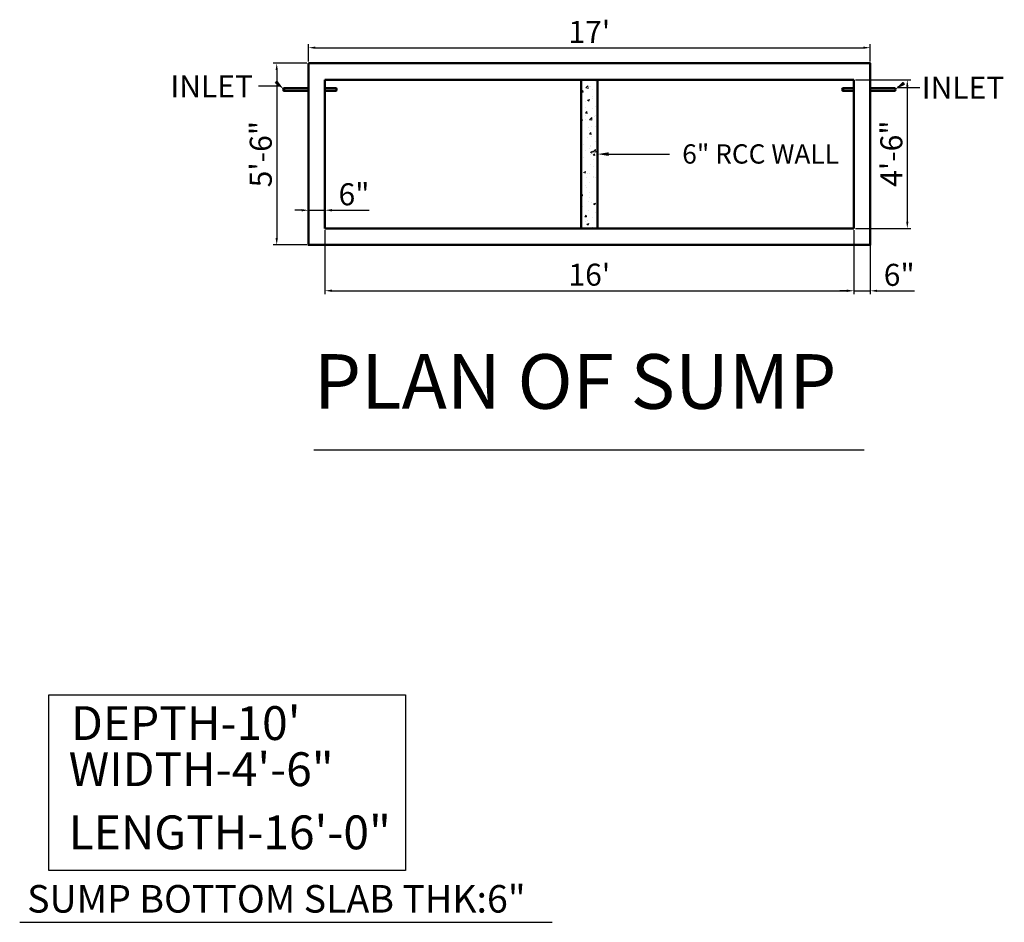
# Model space of a CAD drawing. Units: inches. Extents: x 2473 to 3272, y 1467 to 1853.
# Tile 3 of 3: x 2914 to 3272, y 1505 to 1833. Entities that reach past the tile are written whole.
import ezdxf
from ezdxf import colors
from ezdxf.entities.mleader import LeaderData, LeaderLine
from ezdxf.math import Vec2, Vec3

# ---------------------------------------------------------------- set-up
doc = ezdxf.new("R2010")
doc.units = ezdxf.units.IN
doc.header["$PDMODE"] = 36
for name, color, linetype, lineweight in [('S-ANNO-DIMS', 2, 'Continuous', 25), ('S-ANNO-TEXT', 7, 'Continuous', 25), ('S-CONC', 7, 'Continuous', 50), ('S-CONC-PATT', 8, 'Continuous', 13)]:
    doc.layers.add(name, color=color, linetype=linetype, lineweight=lineweight)
doc.styles.get("Standard").update_dxf_attribs({"font": '@Yu Gothic UI Semibold.ttf'})
doc.dimstyles.new('ISO-25', dxfattribs={"dimtxt": 8, "dimasz": 2.5, "dimexe": 1.25, "dimexo": 0.625, "dimtad": 1, "dimdec": 1, "dimlunit": 3, "dimtxsty": 'Standard', "dimcen": 2.5, "dimadec": 0, "dimazin": 0, "dimtfac": 1, "dimtdec": 1, "dimtmove": 0, "dimatfit": 3, "dimfxl": 1, "dimarcsym": 0})

# ---------------------------------------------------------------- blocks, each defined once
blk = doc.blocks.new('*D1')
at = {"layer": 'Defpoints', "color": 0, "transparency": 16777216}
for p in [(3019.15, 1817.34), (3007.62, 1751.34), (3019.15, 1751.34)]:
    blk.add_point(p, dxfattribs=at)
at = {"layer": 'S-ANNO-DIMS', "color": 0, "lineweight": -2, "transparency": 16777216}
for p, q in [((3018.52, 1817.34), (3006.37, 1817.34)), ((3007.62, 1814.84), (3007.62, 1753.84)), ((3018.52, 1751.34), (3006.37, 1751.34))]:
    blk.add_line(p, q, dxfattribs=at)
at = {"layer": 'S-ANNO-DIMS', "color": 0, "transparency": 16777216}
for points in [[(3007.2, 1814.84), (3008.04, 1814.84), (3007.62, 1817.34)], [(3007.2, 1753.84), (3008.04, 1753.84), (3007.62, 1751.34)]]:
    blk.add_solid(points, dxfattribs=at)
at = {"layer": 'S-ANNO-DIMS', "color": 0, "transparency": 16777216, "insert": (3002.86, 1784.34), "char_height": 8, "attachment_point": 5, "rotation": 90}
blk.add_mtext('5\'-6"', dxfattribs=at)
blk = doc.blocks.new('*D2')
at = {"layer": 'Defpoints', "color": 0, "transparency": 16777216}
for p in [(3217.15, 1811.34), (3217.15, 1757.34), (3236.62, 1757.34)]:
    blk.add_point(p, dxfattribs=at)
at = {"layer": 'S-ANNO-DIMS', "color": 0, "lineweight": -2, "transparency": 16777216}
for p, q in [((3217.77, 1811.34), (3237.87, 1811.34)), ((3236.62, 1808.84), (3236.62, 1759.84)), ((3217.77, 1757.34), (3237.87, 1757.34))]:
    blk.add_line(p, q, dxfattribs=at)
at = {"layer": 'S-ANNO-DIMS', "color": 0, "transparency": 16777216}
for points in [[(3236.2, 1808.84), (3237.04, 1808.84), (3236.62, 1811.34)], [(3236.2, 1759.84), (3237.04, 1759.84), (3236.62, 1757.34)]]:
    blk.add_solid(points, dxfattribs=at)
at = {"layer": 'S-ANNO-DIMS', "color": 0, "transparency": 16777216, "insert": (3231.86, 1784.52), "char_height": 8, "attachment_point": 5, "rotation": 90}
blk.add_mtext('4\'-6"', dxfattribs=at)
blk = doc.blocks.new('*D3')
at = {"layer": 'Defpoints', "color": 0, "transparency": 16777216}
for p in [(3223.15, 1822.99), (3019.15, 1817.34), (3223.15, 1817.34)]:
    blk.add_point(p, dxfattribs=at)
at = {"layer": 'S-ANNO-DIMS', "color": 0, "lineweight": -2, "transparency": 16777216}
for p, q in [((3019.15, 1817.96), (3019.15, 1824.24)), ((3223.15, 1817.96), (3223.15, 1824.24)), ((3021.65, 1822.99), (3220.65, 1822.99))]:
    blk.add_line(p, q, dxfattribs=at)
at = {"layer": 'S-ANNO-DIMS', "color": 0, "transparency": 16777216}
for points in [[(3021.65, 1823.4), (3021.65, 1822.57), (3019.15, 1822.99)], [(3220.65, 1823.4), (3220.65, 1822.57), (3223.15, 1822.99)]]:
    blk.add_solid(points, dxfattribs=at)
at = {"layer": 'S-ANNO-DIMS', "color": 0, "transparency": 16777216, "insert": (3121.15, 1827.7), "char_height": 8, "attachment_point": 5}
blk.add_mtext("17'", dxfattribs=at)
blk = doc.blocks.new('*D4')
at = {"layer": 'Defpoints', "color": 0, "transparency": 16777216}
for p in [(3019.15, 1763.96), (3019.15, 1757.34), (3025.15, 1757.34)]:
    blk.add_point(p, dxfattribs=at)
at = {"layer": 'S-ANNO-DIMS', "color": 0, "lineweight": -2, "transparency": 16777216}
for p, q in [((3016.65, 1763.96), (3014.15, 1763.96)), ((3019.15, 1757.96), (3019.15, 1765.21)), ((3019.15, 1763.96), (3025.15, 1763.96)), ((3025.15, 1757.96), (3025.15, 1765.21)), ((3027.65, 1763.96), (3041.22, 1763.96))]:
    blk.add_line(p, q, dxfattribs=at)
at = {"layer": 'S-ANNO-DIMS', "color": 0, "transparency": 16777216}
for points in [[(3016.65, 1764.38), (3016.65, 1763.54), (3019.15, 1763.96)], [(3027.65, 1764.38), (3027.65, 1763.54), (3025.15, 1763.96)]]:
    blk.add_solid(points, dxfattribs=at)
at = {"layer": 'S-ANNO-DIMS', "color": 0, "transparency": 16777216, "insert": (3035.68, 1768.72), "char_height": 8, "attachment_point": 5}
blk.add_mtext('6"', dxfattribs=at)
blk = doc.blocks.new('*D5')
at = {"layer": 'Defpoints', "color": 0, "transparency": 16777216}
for p in [(3025.15, 1757.34), (3217.15, 1757.34), (3217.15, 1734.74)]:
    blk.add_point(p, dxfattribs=at)
at = {"layer": 'S-ANNO-DIMS', "color": 0, "lineweight": -2, "transparency": 16777216}
for p, q in [((3025.15, 1756.71), (3025.15, 1733.49)), ((3217.15, 1756.71), (3217.15, 1733.49)), ((3027.65, 1734.74), (3214.65, 1734.74))]:
    blk.add_line(p, q, dxfattribs=at)
at = {"layer": 'S-ANNO-DIMS', "color": 0, "transparency": 16777216}
for points in [[(3027.65, 1735.15), (3027.65, 1734.32), (3025.15, 1734.74)], [(3214.65, 1735.15), (3214.65, 1734.32), (3217.15, 1734.74)]]:
    blk.add_solid(points, dxfattribs=at)
at = {"layer": 'S-ANNO-DIMS', "color": 0, "transparency": 16777216, "insert": (3121.15, 1739.52), "char_height": 8, "attachment_point": 5}
blk.add_mtext("16'", dxfattribs=at)
blk = doc.blocks.new('*D19')
at = {"layer": 'Defpoints', "color": 0, "transparency": 16777216}
for p in [(3217.15, 1757.34), (3223.15, 1757.34), (3223.15, 1734.7)]:
    blk.add_point(p, dxfattribs=at)
at = {"layer": 'S-ANNO-DIMS', "color": 0, "lineweight": -2, "transparency": 16777216}
for p, q in [((3217.15, 1756.71), (3217.15, 1733.45)), ((3223.15, 1756.71), (3223.15, 1733.45)), ((3214.65, 1734.7), (3212.15, 1734.7)), ((3217.15, 1734.7), (3223.15, 1734.7)), ((3225.65, 1734.7), (3239.22, 1734.7))]:
    blk.add_line(p, q, dxfattribs=at)
at = {"layer": 'S-ANNO-DIMS', "color": 0, "transparency": 16777216}
for points in [[(3214.65, 1735.11), (3214.65, 1734.28), (3217.15, 1734.7)], [(3225.65, 1735.11), (3225.65, 1734.28), (3223.15, 1734.7)]]:
    blk.add_solid(points, dxfattribs=at)
at = {"layer": 'S-ANNO-DIMS', "color": 0, "transparency": 16777216, "insert": (3233.68, 1739.46), "char_height": 8, "attachment_point": 5}
blk.add_mtext('6"', dxfattribs=at)

msp = doc.modelspace()

# ---------------------------------------------------------------- hatches: boundary and pattern name
at = {"layer": 'S-CONC-PATT'}
h = msp.add_hatch(dxfattribs=at)
h.set_pattern_fill('AR-CONC', color=256, scale=0.04)
h.set_pattern_definition([(50, (440.186, 311.7825), (7.287387, -0.637563), [0.762, -8.382]), (355, (440.186, 311.7825), (-1.409737, 7.642274), [0.6096, -6.705623]), (100.45144, (440.793, 311.729), (5.87765, 7.00471), [0.6476, -7.12361]), (46.1842, (440.186, 313.8145), (10.843162, -1.681693), [1.143, -12.573]), (96.63556, (441.089, 313.674), (9.496165, 9.897045), [0.9714, -10.685424]), (351.18415, (440.186, 313.814), (9.496165, 9.897045), [0.9144, -10.05839]), (21, (441.202, 313.3065), (6.064576, -4.090608), [0.762, -8.382]), (326, (441.202, 313.3065), (2.472081, 7.367519), [0.6096, -6.7056]), (71.45144, (441.707, 312.9656), (8.536657, 3.27691), [0.6476, -7.123598]), (37.5, (440.1859, 311.7825), (0.1235441, 3.3822016), [0, -6.62432, 0, -6.8072, 0, -6.731]), (7.5, (440.186, 311.7825), (2.6727865, 4.007223), [0, -3.88112, 0, -6.47192, 0, -2.5654]), (327.5, (437.9202, 311.7825), (5.4236238, -0.2291498), [0, -2.54, 0, -7.9248, 0, -10.5156]), (317.5, (436.904, 311.7825), (5.925167, 1.01706), [0, -3.302, 0, -5.26288, 0, -7.4676])])
h.paths.add_polyline_path([(3124.15, 1811.34), (3118.15, 1811.34), (3118.15, 1757.34), (3124.15, 1757.34)])

# ---------------------------------------------------------------- linework, layer by layer
at = {"layer": 'S-ANNO-TEXT'}
for p, q in [((3021.13, 1677.01), (3220.98, 1677.01)), ((2914.28, 1505.39), (3107.63, 1505.39))]:
    msp.add_line(p, q, dxfattribs=at)
msp.add_lwpolyline([(2924.9, 1587.96), (3054.33, 1587.96), (3054.33, 1524.19), (2924.9, 1524.19)], close=True, dxfattribs=at)
at = {"layer": 'S-CONC'}
for p, q in [((3025.15, 1811.34), (3217.15, 1811.34)), ((3025.15, 1757.34), (3025.15, 1811.34)), ((3025.15, 1811.34), (3025.15, 1808.34)), ((3118.15, 1757.34), (3118.15, 1811.34)), ((3124.15, 1757.34), (3124.15, 1811.34)), ((3217.15, 1811.34), (3217.15, 1757.34)), ((3010.15, 1808.34), (3019.15, 1808.34)), ((3019.15, 1807.34), (3010.15, 1807.34)), ((3025.15, 1808.34), (3029.15, 1808.34)), ((3029.15, 1807.34), (3025.15, 1807.34)), ((3217.15, 1808.34), (3213.15, 1808.34)), ((3213.15, 1807.34), (3217.15, 1807.34)), ((3232.15, 1808.34), (3223.15, 1808.34)), ((3223.15, 1807.34), (3232.15, 1807.34)), ((3217.15, 1757.34), (3025.15, 1757.34))]:
    msp.add_line(p, q, dxfattribs=at)
msp.add_lwpolyline([(3019.15, 1817.34), (3223.15, 1817.34), (3223.15, 1751.34), (3019.15, 1751.34)], close=True, dxfattribs=at)
for centre in [(3010.15, 1807.84), (3029.15, 1807.84)]:
    msp.add_ellipse(centre, major_axis=(0, 0.5), ratio=0.337525, dxfattribs=at)
at = {"layer": 'S-CONC', "extrusion": (0, 0, -1)}
for centre in [(3213.15, 1807.84), (3232.15, 1807.84)]:
    msp.add_ellipse(centre, major_axis=(0, 0.5), ratio=0.337525, dxfattribs=at)

# ---------------------------------------------------------------- texts
at = {"layer": 'S-ANNO-TEXT'}
for s, height, p in [('PLAN OF SUMP', 19.838, (3021.14, 1691.86)), ("DEPTH-10'", 12.283, (2932.95, 1571.59)), ('WIDTH-4\'-6"', 12.283, (2932.07, 1554.85)), ('LENGTH-16\'-0"', 12.283, (2932.07, 1531.91)), ('SUMP BOTTOM SLAB THK:6"', 10, (2916.99, 1508.92))]:
    msp.add_text(s, height=height, dxfattribs=at).set_placement(p)

# ---------------------------------------------------------------- dimensions: what is measured, and where the dimension line sits
at = {"layer": 'S-ANNO-DIMS'}
for base, p1, p2, override, picture, middle in [((3223.15, 1822.99), (3019.15, 1817.34), (3223.15, 1817.34), {"dimtxt": 8, "dimclrd": 0, "dimclre": 0, "dimclrt": 0}, '*D3', (3121.15, 1827.7)), ((3217.15, 1734.74), (3025.15, 1757.34), (3217.15, 1757.34), {"dimclrd": 0, "dimclre": 0, "dimclrt": 0}, '*D5', (3121.15, 1739.52)), ((3223.15, 1734.7), (3217.15, 1757.34), (3223.15, 1757.34), {"dimclrd": 0, "dimclre": 0, "dimclrt": 0}, '*D19', (3233.68, 1739.46))]:
    dim = msp.add_linear_dim(base=base, p1=p1, p2=p2, dimstyle='ISO-25', override=override, dxfattribs=at)
    dim.commit()
    dim.dimension.update_dxf_attribs({"geometry": picture, "text_midpoint": middle})
dim = msp.add_linear_dim(base=(3007.62, 1751.34), p1=(3019.15, 1817.34), p2=(3019.15, 1751.34), angle=90, dimstyle='ISO-25', override={"dimtxt": 8, "dimclrd": 0, "dimclre": 0, "dimclrt": 0}, dxfattribs=at)
dim.commit()
dim.dimension.update_dxf_attribs({"geometry": '*D1', "text_midpoint": (3002.86, 1784.34)})
dim = msp.add_linear_dim(base=(3236.62, 1757.34), p1=(3217.15, 1811.34), p2=(3217.15, 1757.34), angle=90, dimstyle='ISO-25', override={"dimtxt": 8, "dimclrd": 0, "dimclre": 0, "dimclrt": 0}, dxfattribs=at)
dim.commit()
dim.dimension.update_dxf_attribs({"geometry": '*D2', "text_midpoint": (3236.62, 1784.52), "dimtype": 160})
dim = msp.add_linear_dim(base=(3019.15, 1763.96), p1=(3025.15, 1757.34), p2=(3019.15, 1757.34), dimstyle='ISO-25', override={"dimclrd": 0, "dimclre": 0, "dimclrt": 0}, dxfattribs=at)
dim.commit()
dim.dimension.update_dxf_attribs({"geometry": '*D4', "text_midpoint": (3035.68, 1763.96), "dimtype": 160})

# ---------------------------------------------------------------- leaders
at = {"layer": 'S-ANNO-TEXT'}
ml = msp.add_multileader_mtext('Standard', dxfattribs=at)
ml.set_content('INLET', color=(175, 217, 170))
ml.set_leader_properties()
ml.build(insert=Vec2(0, 0))
ctx = ml.context
ctx.base_point, ctx.char_height, ctx.plane_origin = Vec3(2968.26, 1809), 8, Vec3(3010.15, 1807.84)
ctx.text_align_type = 2
notes = []
notes.append((ctx, [(0, (1, 1, 0), (3008.99, 1809), (-1, 0), 8, [(0, [(3010.15, 1807.84)], 0, [])])]))
ctx.mtext.insert, ctx.mtext.alignment, ctx.mtext.flow_direction = Vec3(2998.99, 1813), 3, 5
ml = msp.add_multileader_mtext('Standard', dxfattribs=at)
ml.set_content('INLET', color=(175, 217, 170))
ml.set_leader_properties()
ml.build(insert=Vec2(0, 0))
ctx = ml.context
ctx.base_point, ctx.char_height, ctx.plane_origin = Vec3(3241.12, 1808.51), 8, Vec3(3232.15, 1807.84)
ctx.text_align_type = 2
notes.append((ctx, [(0, (1, 1, 0), (3233.12, 1808.51), (1, 0), 8, [(0, [(3232.15, 1807.84)], 0, [])])]))
ctx.mtext.insert, ctx.mtext.width, ctx.mtext.alignment, ctx.mtext.flow_direction = Vec3(3271.85, 1812.51), 20, 3, 5
ml = msp.add_multileader_mtext('Standard', dxfattribs=at)
ml.set_content('6" RCC WALL', color=(175, 217, 170))
ml.set_leader_properties()
ml.build(insert=Vec2(0, 0))
ctx = ml.context
ctx.base_point, ctx.char_height, ctx.plane_origin = Vec3(3150.21, 1784.34), 7, Vec3(3124.15, 1784.34)
ctx.text_align_type = 2
notes.append((ctx, [(0, (1, 1, 0), (3142.21, 1784.34), (1, 0), 8, [(0, [(3124.15, 1784.34)], 0, [])])]))
ctx.mtext.insert, ctx.mtext.alignment, ctx.mtext.flow_direction = Vec3(3211.8, 1787.9), 3, 5
for ctx, leaders in notes:
    for number, flags, end, landing, length, lines in leaders:
        leader = LeaderData()
        leader.index, (leader.has_last_leader_line, leader.has_dogleg_vector, leader.attachment_direction) = number, flags
        leader.last_leader_point, leader.dogleg_vector, leader.dogleg_length = Vec3(end), Vec3(landing), length
        for number, points, colour, breaks in lines:
            line = LeaderLine()
            line.index, line.vertices, line.color, line.breaks = number, Vec3.list(points), colors.encode_raw_color(colour), breaks
            leader.lines.append(line)
        ctx.leaders.append(leader)

doc.saveas('drawing.dxf')
